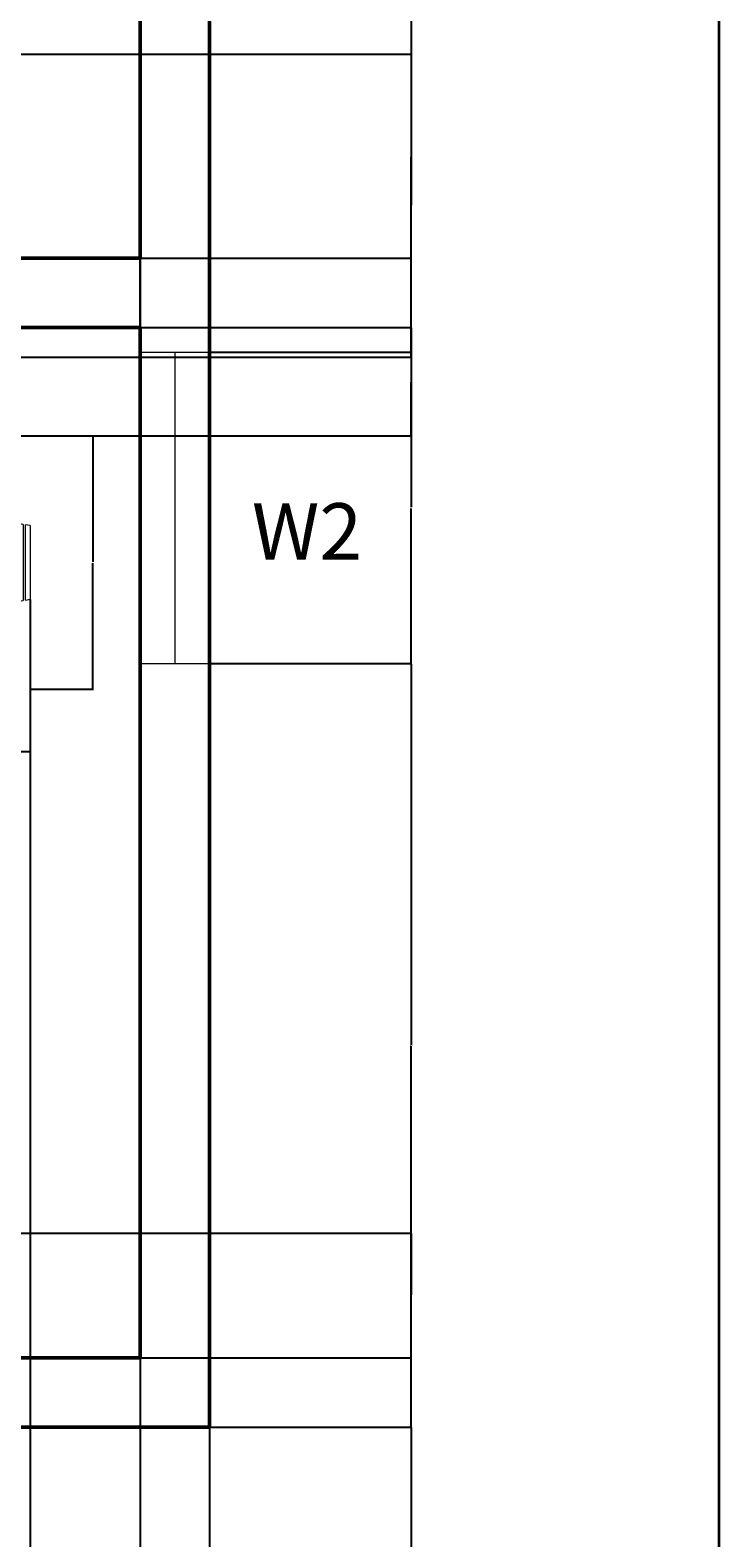
# Model space of a CAD drawing. Units: centimetres. Extents: x 2050 to 3144, y 831 to 2296.
# Tile 5 of 7: x 2916 to 3144, y 1152 to 1650. Entities that reach past the tile are written whole.
import ezdxf

# ---------------------------------------------------------------- set-up
doc = ezdxf.new("R2010")
doc.units = ezdxf.units.CM
for name, color, linetype, lineweight in [('A-ANNO-DIMS', 2, 'Continuous', 18), ('A-ANNO-TEXT', 7, 'Continuous', 18), ('A-ANNO-TTLB', 7, 'Continuous', 35), ('A-FLOR', 7, 'Continuous', 25), ('A-FURN', 8, 'Continuous', 18), ('A-GLAZ', 4, 'Continuous', 18), ('A-WALL', 7, 'Continuous', 50)]:
    doc.layers.add(name, color=color, linetype=linetype, lineweight=lineweight)
doc.styles.get("Standard").update_dxf_attribs({"font": 'arial.ttf'})
doc.dimstyles.get("Standard").update_dxf_attribs({"dimtxt": 0.18, "dimasz": 0.18, "dimexe": 0.18, "dimexo": 0.0625, "dimgap": 0.09, "dimtad": 0, "dimtih": 1, "dimtoh": 1, "dimdec": 4, "dimzin": 0, "dimdsep": 46, "dimtxsty": 'Standard', "dimcen": 0.09, "dimadec": 0, "dimazin": 0, "dimtfac": 1, "dimtdec": 4, "dimtofl": 0, "dimtmove": 0, "dimatfit": 3, "dimfxl": 1, "dimtolj": 1, "dimtzin": 0, "dimarcsym": 0})

# ---------------------------------------------------------------- blocks, each defined once
blk = doc.blocks.new('Dining Set - 36 x 72 in.')
for p, q in [((-22, 27.5), (-22.1562, 26.50042)), ((-5.8416, 26.5), (-22.1534, 26.5)), ((-22, 27.5), (-6, 27.5)), ((-5.8437, 26.49966), (-6, 27.5)), ((6, 27.5), (5.8438, 26.50042)), ((22.1584, 26.5), (5.8466, 26.5)), ((6, 27.5), (22, 27.5)), ((22.1563, 26.49966), (22, 27.5)), ((-22.2343, 26.00059), (-23.4847, 17.99762)), ((-22.2304, 26), (-5.7608, 26)), ((-4.5152, 17.99762), (-5.7655, 25.99926)), ((5.7657, 26.00059), (4.5153, 17.99762)), ((5.7696, 26), (22.2392, 26)), ((23.4848, 17.99762), (22.2345, 25.99926)), ((36, 18), (-36, 18)), ((-36, 18), (-36, -18)), ((36, -18), (36, 18)), ((-45.5, 8), (-44.5004, 8.15617)), ((-45.5, 8), (-45.5, -8)), ((-44.5, -8.15843), (-44.5, 8.15338)), ((-44.0006, 8.23428), (-35.9976, 9.48474)), ((-44, 8.23041), (-44, -8.23915)), ((44.0006, 8.23428), (35.9976, 9.48474)), ((44, 8.23041), (44, -8.23915)), ((44.5, -8.15843), (44.5, 8.15338)), ((45.5, 8), (44.5005, 8.15617)), ((45.5, 8), (45.5, -8)), ((-44.4997, -8.15631), (-45.5, -8)), ((-35.9976, -9.48476), (-43.9993, -8.2345)), ((35.9976, -9.48476), (43.9993, -8.2345)), ((44.4997, -8.15631), (45.5, -8)), ((-36, -18), (36, -18)), ((-22.2343, -26.0006), (-23.4847, -17.99762)), ((-4.5152, -17.99762), (-5.7655, -25.99928)), ((5.7657, -26.0006), (4.5153, -17.99762)), ((23.4848, -17.99762), (22.2345, -25.99928)), ((-22.2304, -26), (-5.7608, -26)), ((5.7696, -26), (22.2392, -26)), ((-22, -27.5), (-22.1562, -26.50044)), ((-5.8416, -26.5), (-22.1534, -26.5)), ((-22, -27.5), (-6, -27.5)), ((-5.8437, -26.49967), (-6, -27.5)), ((6, -27.5), (5.8438, -26.50044)), ((22.1584, -26.5), (5.8466, -26.5)), ((6, -27.5), (22, -27.5)), ((22.1563, -26.49967), (22, -27.5))]:
    blk.add_line(p, q)
for points in [[(-36, 15), (-31.1772, 14.97754), (-26.8079, 14.91406), (-22.8538, 14.81543), (-19.276, 14.6875), (-16.0362, 14.53613), (-13.0957, 14.36718), (-10.4159, 14.18652), (-7.9583, 14), (-5.6904, 13.81315), (-3.6035, 13.63021), (-1.6954, 13.45508), (0.0365, 13.29166), (1.5945, 13.14388), (2.9811, 13.01562), (4.1988, 12.9108), (5.25, 12.83333), (6.1393, 12.78613), (6.8802, 12.76823), (7.4883, 12.77767), (7.9792, 12.8125), (8.3685, 12.87077), (8.6719, 12.95052), (8.9049, 13.0498), (9.0833, 13.16666), (9.2205, 13.29899), (9.3216, 13.44401), (9.3895, 13.59879), (9.4271, 13.76041), (9.4373, 13.92594), (9.4232, 14.09245), (9.3875, 14.257), (9.3333, 14.41666), (9.2638, 14.56917), (9.1836, 14.71484), (9.0975, 14.85465), (9.0104, 14.98958), (8.9272, 15.1206), (8.8529, 15.2487), (8.7922, 15.37483), (8.75, 15.5), (8.7305, 15.62467), (8.7344, 15.74739), (8.7617, 15.86621), (8.8125, 15.97916), (8.8867, 16.08431), (8.9844, 16.17968), (9.1055, 16.26334), (9.25, 16.33333), (9.4189, 16.38802), (9.6172, 16.42708), (9.8506, 16.45052), (10.125, 16.45833), (10.4463, 16.45052), (10.8203, 16.42708), (11.2529, 16.38802), (11.75, 16.33333), (12.3184, 16.26318), (12.9694, 16.17838), (13.7151, 16.07991), (14.5677, 15.96875), (15.5395, 15.84586), (16.6426, 15.71224), (17.8893, 15.56884), (19.2917, 15.41666), (20.859, 15.25667), (22.5879, 15.08984), (24.4721, 14.91715), (26.5052, 14.73958), (28.6809, 14.5581), (30.9929, 14.3737), (33.4347, 14.18733), (36, 14)], [(-36, 10), (-28.9766, 10.14274), (-23.1725, 10.20442), (-18.4241, 10.19775), (-14.5677, 10.13541), (-11.4399, 10.03011), (-8.877, 9.89453), (-6.7154, 9.74137), (-4.7917, 9.58333), (-2.9698, 9.43082), (-1.2246, 9.28515), (0.4415, 9.14534), (2.026, 9.01041), (3.5266, 8.87939), (4.9408, 8.7513), (6.266, 8.62516), (7.5, 8.5), (8.6411, 8.37549), (9.6914, 8.2539), (10.6538, 8.13818), (11.5312, 8.03125), (12.3267, 7.93603), (13.043, 7.85547), (13.6831, 7.79248), (14.25, 7.75), (14.7471, 7.7303), (15.1797, 7.73307), (15.5537, 7.75732), (15.875, 7.80208), (16.1494, 7.86637), (16.3828, 7.94922), (16.5811, 8.04964), (16.75, 8.16666), (16.8944, 8.29915), (17.0143, 8.44531), (17.1089, 8.60319), (17.1771, 8.77083), (17.218, 8.94629), (17.2305, 9.1276), (17.2137, 9.31282), (17.1667, 9.5), (17.0895, 9.6875), (16.987, 9.875), (16.8649, 10.0625), (16.7292, 10.25), (16.5856, 10.4375), (16.4401, 10.625), (16.2985, 10.8125), (16.1667, 11), (16.05, 11.18733), (15.9518, 11.3737), (15.8752, 11.5581), (15.8229, 11.73958), (15.798, 11.91715), (15.8034, 12.08984), (15.842, 12.25667), (15.9167, 12.41666), (16.0295, 12.56836), (16.1784, 12.70833), (16.3605, 12.83268), (16.5729, 12.9375), (16.8127, 13.01888), (17.0768, 13.07291), (17.3625, 13.0957), (17.6667, 13.08333), (17.9894, 13.03312), (18.3418, 12.94726), (18.7382, 12.82918), (19.1927, 12.68229), (19.7195, 12.51001), (20.3327, 12.31575), (21.0465, 12.10294), (21.875, 11.875), (22.8357, 11.63354), (23.959, 11.37304), (25.2786, 11.08618), (26.8282, 10.76562), (28.6414, 10.40405), (30.752, 9.99414), (33.1936, 9.52856), (36, 9)], [(-36, 5.5), (-30.7157, 5.3348), (-26.069, 5.20963), (-21.9946, 5.11767), (-18.4271, 5.05208), (-15.3009, 5.00602), (-12.5508, 4.97265), (-10.1112, 4.94515), (-7.9167, 4.91666), (-5.909, 4.88167), (-4.0586, 4.83984), (-2.3429, 4.79215), (-0.7396, 4.73958), (0.7739, 4.6831), (2.22, 4.6237), (3.6213, 4.56233), (5, 4.5), (6.373, 4.43782), (7.7344, 4.3776), (9.0723, 4.32129), (10.375, 4.27083), (11.6309, 4.22819), (12.8281, 4.19531), (13.9551, 4.17415), (15, 4.16666), (15.954, 4.17448), (16.819, 4.19791), (17.6001, 4.23698), (18.3021, 4.29166), (18.9299, 4.36198), (19.4883, 4.44791), (19.9823, 4.54948), (20.4167, 4.66666), (20.7969, 4.79899), (21.1302, 4.94401), (21.4245, 5.09879), (21.6875, 5.26041), (21.9271, 5.42594), (22.1511, 5.59245), (22.3672, 5.757), (22.5834, 5.91666), (22.8065, 6.06868), (23.0404, 6.21093), (23.2879, 6.34147), (23.5521, 6.45833), (23.8358, 6.55957), (24.142, 6.64323), (24.4735, 6.70735), (24.8334, 6.75), (25.2235, 6.76969), (25.642, 6.76692), (26.0858, 6.74267), (26.5521, 6.69791), (27.0379, 6.63362), (27.5404, 6.55078), (28.0565, 6.45036), (28.5834, 6.33333), (29.1242, 6.19987), (29.7071, 6.04687), (30.3661, 5.87044), (31.1354, 5.66666), (32.0493, 5.43164), (33.142, 5.16146), (34.4475, 4.85221), (36, 4.5)], [(-36, -1), (-30.7915, -0.6591), (-26.0195, -0.38216), (-21.6519, -0.16284), (-17.6563, 0.00521), (-14.0005, 0.12833), (-10.6523, 0.21289), (-7.5796, 0.26522), (-4.75, 0.29166), (-2.134, 0.29793), (0.2878, 0.28711), (2.5317, 0.26163), (4.6146, 0.22396), (6.5529, 0.17651), (8.3633, 0.12174), (10.0623, 0.06209), (11.6667, 0), (13.1899, -0.06201), (14.6341, -0.1211), (15.9982, -0.17432), (17.2813, -0.21875), (18.4823, -0.25147), (19.6003, -0.26953), (20.6343, -0.27002), (21.5834, -0.25), (22.4481, -0.20768), (23.2357, -0.14584), (23.9549, -0.06836), (24.6146, 0.02083), (25.2235, 0.11784), (25.7904, 0.21875), (26.3241, 0.31966), (26.8334, 0.41666), (27.3265, 0.50618), (27.8099, 0.58593), (28.2894, 0.65397), (28.7709, 0.70833), (29.2601, 0.74707), (29.763, 0.76823), (30.2855, 0.76985), (30.8334, 0.75), (31.4088, 0.70784), (31.9994, 0.64713), (32.589, 0.57275), (33.1615, 0.48958), (33.7008, 0.4025), (34.1908, 0.3164), (34.6153, 0.23616), (34.9584, 0.16666), (35.2099, 0.11165), (35.3848, 0.07031), (35.504, 0.04069), (35.5886, 0.02083), (35.6594, 0.00879), (35.7377, 0.0026), (35.8442, 0.00032), (36, 0)], [(-36, -6.5), (-27.1843, -6.31267), (-20.084, -6.1263), (-14.469, -5.9419), (-10.1094, -5.76042), (-6.7752, -5.58285), (-4.2363, -5.41016), (-2.2629, -5.24333), (-0.625, -5.08334), (0.8708, -4.93099), (2.2715, -4.78646), (3.5872, -4.64974), (4.8281, -4.52084), (6.0046, -4.39974), (7.127, -4.28646), (8.2053, -4.18099), (9.25, -4.08334), (10.2705, -3.99382), (11.2734, -3.91407), (12.2647, -3.84603), (13.25, -3.79167), (14.2354, -3.75293), (15.2266, -3.73177), (16.2295, -3.73015), (17.25, -3.75), (18.2912, -3.79248), (19.3451, -3.85547), (20.4009, -3.93604), (21.4479, -4.03125), (22.4754, -4.13819), (23.4727, -4.25391), (24.4289, -4.37549), (25.3334, -4.5), (26.1785, -4.62492), (26.9694, -4.74935), (27.7145, -4.87281), (28.4219, -4.99479), (29.1, -5.11483), (29.7572, -5.23242), (30.4016, -5.34709), (31.0417, -5.45834), (31.6837, -5.56437), (32.3262, -5.65821), (32.9658, -5.73153), (33.599, -5.77604), (34.2224, -5.78345), (34.8327, -5.74545), (35.4264, -5.65373), (36, -5.5)], [(-36, -10), (-26.4022, -9.81299), (-18.4675, -9.62891), (-11.9839, -9.45069), (-6.7396, -9.28125), (-2.5226, -9.12354), (0.8789, -8.98047), (3.6769, -8.85498), (6.0833, -8.75), (8.2767, -8.66765), (10.3021, -8.60677), (12.1712, -8.56543), (13.8958, -8.54167), (15.4876, -8.53353), (16.9583, -8.53907), (18.3197, -8.55632), (19.5834, -8.58334), (20.7616, -8.61841), (21.8685, -8.66081), (22.9188, -8.71004), (23.9271, -8.76563), (24.9081, -8.82707), (25.8763, -8.89388), (26.8465, -8.96558), (27.8334, -9.04167), (28.8474, -9.12118), (29.8828, -9.20117), (30.93, -9.27824), (31.9792, -9.34896), (33.0205, -9.40991), (34.0443, -9.45768), (35.0407, -9.48885), (36, -9.5)], [(-36, -14.5), (-30.0881, -14.33513), (-25.0332, -14.21224), (-20.7312, -14.12647), (-17.0781, -14.07292), (-13.97, -14.04671), (-11.3027, -14.04297), (-8.9724, -14.05681), (-6.875, -14.08334), (-4.9224, -14.11833), (-3.0905, -14.16016), (-1.3709, -14.20785), (0.2448, -14.26042), (1.7647, -14.3169), (3.1973, -14.3763), (4.5507, -14.43767), (5.8333, -14.5), (7.0554, -14.5621), (8.235, -14.62175), (9.3922, -14.67652), (10.5469, -14.72396), (11.7192, -14.76164), (12.929, -14.78711), (14.1965, -14.79794), (15.5417, -14.79167), (16.9933, -14.76424), (18.6152, -14.70508), (20.4804, -14.60197), (22.6615, -14.44271), (25.2312, -14.21509), (28.2624, -13.9069), (31.8277, -13.50594), (36, -13)]]:
    blk.add_lwpolyline(points)
blk = doc.blocks.new('*D19')
at = {"layer": 'A-ANNO-DIMS', "color": 0, "lineweight": -2, "transparency": 16777216}
for p, q in [((2778.22, 1432.48), (2778.22, 1411.63)), ((2916.44, 1432.48), (2916.44, 1411.63)), ((2778.4, 1411.81), (2846.29, 1411.81)), ((2916.26, 1411.81), (2848.37, 1411.81))]:
    blk.add_line(p, q, dxfattribs=at)
at = {"layer": 'A-ANNO-DIMS', "color": 0, "transparency": 16777216}
for points in [[(2778.4, 1411.84), (2778.4, 1411.78), (2778.22, 1411.81)], [(2916.26, 1411.84), (2916.26, 1411.78), (2916.44, 1411.81)]]:
    blk.add_solid(points, dxfattribs=at)
at = {"layer": 'Defpoints', "color": 0, "transparency": 16777216}
for p in [(2778.22, 1432.54), (2916.44, 1432.54), (2916.44, 1411.81)]:
    blk.add_point(p, dxfattribs=at)
at = {"layer": 'A-ANNO-DIMS', "color": 0, "transparency": 16777216, "insert": (2847.33, 1411.81), "char_height": 0.18, "attachment_point": 5}
blk.add_mtext('\\A1;DINING SET 138', dxfattribs=at)
blk = doc.blocks.new('*D20')
at = {"layer": 'A-ANNO-DIMS', "color": 0, "lineweight": -2, "transparency": 16777216}
for p, q in [((2916.5, 1516.08), (2937.35, 1516.08)), ((2937.17, 1515.9), (2937.17, 1474.49)), ((2937.17, 1432.72), (2937.17, 1474.13)), ((2916.5, 1432.54), (2937.35, 1432.54))]:
    blk.add_line(p, q, dxfattribs=at)
at = {"layer": 'A-ANNO-DIMS', "color": 0, "transparency": 16777216}
for points in [[(2937.14, 1515.9), (2937.2, 1515.9), (2937.17, 1516.08)], [(2937.14, 1432.72), (2937.2, 1432.72), (2937.17, 1432.54)]]:
    blk.add_solid(points, dxfattribs=at)
at = {"layer": 'Defpoints', "color": 0, "transparency": 16777216}
for p in [(2916.44, 1516.08), (2937.17, 1516.08), (2916.44, 1432.54)]:
    blk.add_point(p, dxfattribs=at)
at = {"layer": 'A-ANNO-DIMS', "color": 0, "transparency": 16777216, "insert": (2937.17, 1474.31), "char_height": 0.18, "attachment_point": 5}
blk.add_mtext('\\A1;84', dxfattribs=at)
blk = doc.blocks.new('*D43')
at = {"layer": 'A-ANNO-DIMS', "color": 0, "lineweight": -2, "transparency": 16777216}
for p, q in [((2975.65, 1440.94), (3042.37, 1440.94)), ((3042.19, 1440.76), (3042.19, 1315.16)), ((3042.19, 1189.19), (3042.19, 1314.8)), ((2975.65, 1189.01), (3042.37, 1189.01))]:
    blk.add_line(p, q, dxfattribs=at)
at = {"layer": 'A-ANNO-DIMS', "color": 0, "transparency": 16777216}
for points in [[(3042.16, 1440.76), (3042.22, 1440.76), (3042.19, 1440.94)], [(3042.16, 1189.19), (3042.22, 1189.19), (3042.19, 1189.01)]]:
    blk.add_solid(points, dxfattribs=at)
at = {"layer": 'Defpoints', "color": 0, "transparency": 16777216}
for p in [(2975.59, 1440.94), (3042.19, 1440.94), (2975.59, 1189.01)]:
    blk.add_point(p, dxfattribs=at)
at = {"layer": 'A-ANNO-DIMS', "color": 0, "transparency": 16777216, "insert": (3042.19, 1314.98), "char_height": 0.18, "attachment_point": 5}
blk.add_mtext('\\A1;251.93', dxfattribs=at)
blk = doc.blocks.new('*D44')
at = {"layer": 'A-ANNO-DIMS', "color": 0, "lineweight": -2, "transparency": 16777216}
for p, q in [((2975.65, 1543.76), (3042.37, 1543.76)), ((3042.19, 1543.58), (3042.19, 1492.53)), ((3042.19, 1441.12), (3042.19, 1492.17)), ((2975.65, 1440.94), (3042.37, 1440.94))]:
    blk.add_line(p, q, dxfattribs=at)
at = {"layer": 'A-ANNO-DIMS', "color": 0, "transparency": 16777216}
for points in [[(3042.16, 1543.58), (3042.22, 1543.58), (3042.19, 1543.76)], [(3042.16, 1441.12), (3042.22, 1441.12), (3042.19, 1440.94)]]:
    blk.add_solid(points, dxfattribs=at)
at = {"layer": 'Defpoints', "color": 0, "transparency": 16777216}
for p in [(2975.59, 1543.76), (3042.19, 1543.76), (2975.59, 1440.94)]:
    blk.add_point(p, dxfattribs=at)
at = {"layer": 'A-ANNO-DIMS', "color": 0, "transparency": 16777216, "insert": (3042.19, 1492.35), "char_height": 0.18, "attachment_point": 5}
blk.add_mtext('\\A1;102.81', dxfattribs=at)
blk = doc.blocks.new('*D45')
at = {"layer": 'A-ANNO-DIMS', "color": 0, "lineweight": -2, "transparency": 16777216}
for p, q in [((2975.65, 1663.11), (3042.37, 1663.11)), ((3042.19, 1662.93), (3042.19, 1603.62)), ((3042.19, 1543.94), (3042.19, 1603.25)), ((2975.65, 1543.76), (3042.37, 1543.76))]:
    blk.add_line(p, q, dxfattribs=at)
at = {"layer": 'A-ANNO-DIMS', "color": 0, "transparency": 16777216}
for points in [[(3042.16, 1662.93), (3042.22, 1662.93), (3042.19, 1663.11)], [(3042.16, 1543.94), (3042.22, 1543.94), (3042.19, 1543.76)]]:
    blk.add_solid(points, dxfattribs=at)
at = {"layer": 'Defpoints', "color": 0, "transparency": 16777216}
for p in [(2975.59, 1663.11), (3042.19, 1663.11), (2975.59, 1543.76)]:
    blk.add_point(p, dxfattribs=at)
at = {"layer": 'A-ANNO-DIMS', "color": 0, "transparency": 16777216, "insert": (3042.19, 1603.43), "char_height": 0.18, "attachment_point": 5}
blk.add_mtext('\\A1;119.36', dxfattribs=at)
blk = doc.blocks.new('*D52')
at = {"layer": 'A-ANNO-DIMS', "color": 0, "lineweight": -2, "transparency": 16777216}
for p, q in [((2513.42, 1642.03), (3042.37, 1642.03)), ((3042.19, 1641.85), (3042.19, 1592.22)), ((3042.19, 1542.21), (3042.19, 1591.85)), ((2513.42, 1542.03), (3042.37, 1542.03))]:
    blk.add_line(p, q, dxfattribs=at)
at = {"layer": 'A-ANNO-DIMS', "color": 0, "transparency": 16777216}
for points in [[(3042.16, 1641.85), (3042.22, 1641.85), (3042.19, 1642.03)], [(3042.16, 1542.21), (3042.22, 1542.21), (3042.19, 1542.03)]]:
    blk.add_solid(points, dxfattribs=at)
at = {"layer": 'Defpoints', "color": 0, "transparency": 16777216}
for p in [(2513.36, 1642.03), (3042.19, 1642.03), (2513.36, 1542.03)]:
    blk.add_point(p, dxfattribs=at)
at = {"layer": 'A-ANNO-DIMS', "color": 0, "transparency": 16777216, "insert": (3042.19, 1592.03), "char_height": 0.18, "attachment_point": 5}
blk.add_mtext('\\A1;100', dxfattribs=at)
blk = doc.blocks.new('*D56')
at = {"layer": 'A-ANNO-DIMS', "color": 0, "lineweight": -2, "transparency": 16777216}
for p, q in [((2652.79, 1642.03), (3042.37, 1642.03)), ((3042.19, 1641.85), (3042.19, 1608.57)), ((3042.19, 1574.91), (3042.19, 1608.2)), ((2630.24, 1574.73), (3042.37, 1574.73))]:
    blk.add_line(p, q, dxfattribs=at)
at = {"layer": 'A-ANNO-DIMS', "color": 0, "transparency": 16777216}
for points in [[(3042.16, 1641.85), (3042.22, 1641.85), (3042.19, 1642.03)], [(3042.16, 1574.91), (3042.22, 1574.91), (3042.19, 1574.73)]]:
    blk.add_solid(points, dxfattribs=at)
at = {"layer": 'Defpoints', "color": 0, "transparency": 16777216}
for p in [(2652.73, 1642.03), (2630.18, 1574.73), (3042.19, 1574.73)]:
    blk.add_point(p, dxfattribs=at)
at = {"layer": 'A-ANNO-DIMS', "color": 0, "transparency": 16777216, "insert": (3042.19, 1608.38), "char_height": 0.18, "attachment_point": 5}
blk.add_mtext('\\A1;67.3', dxfattribs=at)
blk = doc.blocks.new('*D57')
at = {"layer": 'A-ANNO-DIMS', "color": 0, "lineweight": -2, "transparency": 16777216}
for p, q in [((2916.44, 1462.1), (2916.44, 1009.53)), ((2952.73, 1440.88), (2952.73, 1009.53)), ((2916.62, 1009.71), (2934.19, 1009.71)), ((2952.55, 1009.71), (2934.98, 1009.71))]:
    blk.add_line(p, q, dxfattribs=at)
at = {"layer": 'A-ANNO-DIMS', "color": 0, "transparency": 16777216}
for points in [[(2916.62, 1009.74), (2916.62, 1009.68), (2916.44, 1009.71)], [(2952.55, 1009.74), (2952.55, 1009.68), (2952.73, 1009.71)]]:
    blk.add_solid(points, dxfattribs=at)
at = {"layer": 'Defpoints', "color": 0, "transparency": 16777216}
for p in [(2916.44, 1462.16), (2952.73, 1440.94), (2952.73, 1009.71)]:
    blk.add_point(p, dxfattribs=at)
at = {"layer": 'A-ANNO-DIMS', "color": 0, "transparency": 16777216, "insert": (2934.58, 1009.71), "char_height": 0.18, "attachment_point": 5}
blk.add_mtext('\\A1;36.29', dxfattribs=at)
blk = doc.blocks.new('*D58')
at = {"layer": 'A-ANNO-DIMS', "color": 0, "lineweight": -2, "transparency": 16777216}
for p, q in [((2952.79, 1551.87), (3042.37, 1551.87)), ((3042.19, 1551.69), (3042.19, 1534.16)), ((3042.19, 1516.26), (3042.19, 1533.8)), ((2838.28, 1516.08), (3042.37, 1516.08))]:
    blk.add_line(p, q, dxfattribs=at)
at = {"layer": 'A-ANNO-DIMS', "color": 0, "transparency": 16777216}
for points in [[(3042.16, 1551.69), (3042.22, 1551.69), (3042.19, 1551.87)], [(3042.16, 1516.26), (3042.22, 1516.26), (3042.19, 1516.08)]]:
    blk.add_solid(points, dxfattribs=at)
at = {"layer": 'Defpoints', "color": 0, "transparency": 16777216}
for p in [(2952.73, 1551.87), (3042.19, 1551.87), (2838.22, 1516.08)]:
    blk.add_point(p, dxfattribs=at)
at = {"layer": 'A-ANNO-DIMS', "color": 0, "transparency": 16777216, "insert": (3042.19, 1533.98), "char_height": 0.18, "attachment_point": 5}
blk.add_mtext('\\A1;35.794', dxfattribs=at)
blk = doc.blocks.new('*D59')
at = {"layer": 'A-ANNO-DIMS', "color": 0, "lineweight": -2, "transparency": 16777216}
for p, q in [((2862.15, 1253.11), (2862.15, 2154.53)), ((2862.33, 2154.35), (2907.04, 2154.35)), ((2952.55, 2154.35), (2907.83, 2154.35)), ((2952.73, 1211.94), (2952.73, 2154.53))]:
    blk.add_line(p, q, dxfattribs=at)
at = {"layer": 'A-ANNO-DIMS', "color": 0, "transparency": 16777216}
for points in [[(2862.33, 2154.38), (2862.33, 2154.32), (2862.15, 2154.35)], [(2952.55, 2154.38), (2952.55, 2154.32), (2952.73, 2154.35)]]:
    blk.add_solid(points, dxfattribs=at)
at = {"layer": 'Defpoints', "color": 0, "transparency": 16777216}
for p in [(2952.73, 2154.35), (2862.15, 1253.05), (2952.73, 1211.87)]:
    blk.add_point(p, dxfattribs=at)
at = {"layer": 'A-ANNO-DIMS', "color": 0, "transparency": 16777216, "insert": (2907.44, 2154.35), "char_height": 0.18, "attachment_point": 5}
blk.add_mtext('\\A1;90.58', dxfattribs=at)
blk = doc.blocks.new('*D60')
at = {"layer": 'A-ANNO-DIMS', "color": 0, "lineweight": -2, "transparency": 16777216}
for p, q in [((2862.21, 1253.05), (3042.37, 1253.05)), ((3042.19, 1252.87), (3042.19, 1232.65)), ((3042.19, 1212.05), (3042.19, 1232.28)), ((2895.42, 1211.87), (3042.37, 1211.87))]:
    blk.add_line(p, q, dxfattribs=at)
at = {"layer": 'A-ANNO-DIMS', "color": 0, "transparency": 16777216}
for points in [[(3042.16, 1252.87), (3042.22, 1252.87), (3042.19, 1253.05)], [(3042.16, 1212.05), (3042.22, 1212.05), (3042.19, 1211.87)]]:
    blk.add_solid(points, dxfattribs=at)
at = {"layer": 'Defpoints', "color": 0, "transparency": 16777216}
for p in [(2862.15, 1253.05), (2895.36, 1211.87), (3042.19, 1211.87)]:
    blk.add_point(p, dxfattribs=at)
at = {"layer": 'A-ANNO-DIMS', "color": 0, "transparency": 16777216, "insert": (3042.19, 1232.46), "char_height": 0.18, "attachment_point": 5}
blk.add_mtext('\\A1;41.18', dxfattribs=at)
blk = doc.blocks.new('*D64')
at = {"layer": 'A-ANNO-DIMS', "color": 0, "lineweight": -2, "transparency": 16777216}
for p, q in [((2975.65, 1189.01), (3042.37, 1189.01)), ((3042.19, 1188.83), (3042.19, 1132.85)), ((3042.19, 1076.49), (3042.19, 1132.48)), ((2975.65, 1076.31), (3042.37, 1076.31))]:
    blk.add_line(p, q, dxfattribs=at)
at = {"layer": 'A-ANNO-DIMS', "color": 0, "transparency": 16777216}
for points in [[(3042.16, 1188.83), (3042.22, 1188.83), (3042.19, 1189.01)], [(3042.16, 1076.49), (3042.22, 1076.49), (3042.19, 1076.31)]]:
    blk.add_solid(points, dxfattribs=at)
at = {"layer": 'Defpoints', "color": 0, "transparency": 16777216}
for p in [(2975.59, 1189.01), (3042.19, 1189.01), (2975.59, 1076.31)]:
    blk.add_point(p, dxfattribs=at)
at = {"layer": 'A-ANNO-DIMS', "color": 0, "transparency": 16777216, "insert": (3042.19, 1132.66), "char_height": 0.18, "attachment_point": 5}
blk.add_mtext('\\A1;112.7', dxfattribs=at)
blk = doc.blocks.new('*D74')
at = {"layer": 'A-ANNO-DIMS', "color": 0, "lineweight": -2, "transparency": 16777216}
for p, q in [((2952.73, 2064.83), (2952.73, 1009.53)), ((2822.89, 2004.16), (2822.89, 1009.53)), ((2823.07, 1009.71), (2887.35, 1009.71)), ((2952.55, 1009.71), (2888.26, 1009.71))]:
    blk.add_line(p, q, dxfattribs=at)
at = {"layer": 'A-ANNO-DIMS', "color": 0, "transparency": 16777216}
for points in [[(2823.07, 1009.74), (2823.07, 1009.68), (2822.89, 1009.71)], [(2952.55, 1009.74), (2952.55, 1009.68), (2952.73, 1009.71)]]:
    blk.add_solid(points, dxfattribs=at)
at = {"layer": 'Defpoints', "color": 0, "transparency": 16777216}
for p in [(2952.73, 2064.89), (2822.89, 2004.22), (2952.73, 1009.71)]:
    blk.add_point(p, dxfattribs=at)
at = {"layer": 'A-ANNO-DIMS', "color": 0, "transparency": 16777216, "insert": (2887.81, 1009.71), "char_height": 0.18, "attachment_point": 5}
blk.add_mtext('\\A1;129.84', dxfattribs=at)

msp = doc.modelspace()

# ---------------------------------------------------------------- linework, layer by layer
at = {"layer": 'A-ANNO-TTLB'}
msp.add_lwpolyline([(2050.3641, 2295.8578), (3143.7558, 2295.8578), (3143.7558, 830.6902), (2050.3641, 830.6902)], close=True, dxfattribs=at)
at = {"layer": 'A-FLOR'}
msp.add_line((2975.5865, 1551.8748), (2975.5865, 1076.3148), dxfattribs=at)
at = {"layer": 'A-GLAZ'}
for p, q in [((2952.7265, 1543.7558), (2975.5865, 1543.7558)), ((2964.1565, 1543.7558), (2964.1565, 1440.9424)), ((2952.7265, 1440.9424), (2975.5865, 1440.9424))]:
    msp.add_line(p, q, dxfattribs=at)
at = {"layer": 'A-WALL'}
for p, q in [((2952.7265, 1914.7348), (2952.7265, 1574.7348)), ((2975.5865, 1914.7348), (2975.5865, 1189.0148)), ((2952.7265, 1574.7348), (2629.8665, 1574.7348)), ((2952.7265, 1574.7348), (2952.7265, 1574.7348)), ((2952.7265, 1551.8748), (2629.8665, 1551.8748)), ((2952.7265, 1551.8748), (2952.7265, 1211.8748)), ((2952.7265, 1211.8748), (2669.2319, 1211.8748)), ((2975.5865, 1189.0148), (2669.2319, 1189.0148))]:
    msp.add_line(p, q, dxfattribs=at)

# ---------------------------------------------------------------- block references
at = {"layer": 'A-FURN', "xscale": 1.518878716440213, "yscale": 1.518878716440213, "zscale": 1.518878716440213}
msp.add_blockref('Dining Set - 36 x 72 in.', (2847.3285, 1474.3117), dxfattribs=at)

# ---------------------------------------------------------------- texts
at = {"layer": 'A-ANNO-TEXT'}
msp.add_text('W2', height=18.59595, dxfattribs=at).set_placement((2989.6243, 1475.2678))

# ---------------------------------------------------------------- dimensions: what is measured, and where the dimension line sits
at = {"layer": 'A-ANNO-DIMS'}
for base, p1, p2, picture, middle in [((2952.7265, 2154.3548), (2862.1454, 1253.0515), (2952.7265, 1211.8748), '*D59', (2907.436, 2154.3548)), ((2952.7265, 1009.7148), (2822.8865, 2004.2202), (2952.7265, 2064.8948), '*D74', (2887.8065, 1009.7148)), ((2952.7265, 1009.7148), (2916.4375, 1462.1606), (2952.7265, 1440.9424), '*D57', (2934.582, 1009.7148))]:
    dim = msp.add_linear_dim(base=base, p1=p1, p2=p2, dimstyle='Standard', override={"dimdec": 2, "dimlfac": 1, "dimrnd": 0, "dimzin": 0, "dimdsep": 46, "dimlunit": 2}, dxfattribs=at)
    dim.commit()
    dim.dimension.update_dxf_attribs({"geometry": picture, "text_midpoint": middle})
for base, p1, p2, override, picture, middle in [((3042.1865, 1663.1111), (2975.5865, 1543.7558), (2975.5865, 1663.1111), {"dimdec": 2, "dimlfac": 1, "dimrnd": 0, "dimzin": 0, "dimdsep": 46, "dimlunit": 2}, '*D45', (3042.1865, 1603.4335)), ((3042.1865, 1642.0348), (2513.3612, 1542.0348), (2513.3612, 1642.0348), {"dimdec": 0, "dimlfac": 1, "dimrnd": 0, "dimzin": 0, "dimdsep": 46, "dimlunit": 2}, '*D52', (3042.1865, 1592.0348)), ((3042.1865, 1574.7348), (2652.7265, 1642.0348), (2630.1795, 1574.7348), {"dimdec": 1, "dimlfac": 1, "dimrnd": 0, "dimzin": 0, "dimdsep": 46, "dimlunit": 2}, '*D56', (3042.1865, 1608.3848)), ((3042.1865, 1551.8748), (2838.2153, 1516.0808), (2952.7265, 1551.8748), {"dimdec": 3, "dimlfac": 1, "dimrnd": 0, "dimzin": 0, "dimdsep": 46, "dimlunit": 2}, '*D58', (3042.1865, 1533.9778)), ((3042.1865, 1543.7558), (2975.5865, 1440.9424), (2975.5865, 1543.7558), {"dimdec": 2, "dimlfac": 1, "dimrnd": 0, "dimzin": 0, "dimdsep": 46, "dimlunit": 2}, '*D44', (3042.1865, 1492.3491)), ((2937.1702, 1516.0808), (2916.4375, 1432.5425), (2916.4375, 1516.0808), {"dimdec": 0, "dimlfac": 1, "dimrnd": 0, "dimzin": 0, "dimdsep": 46, "dimlunit": 2}, '*D20', (2937.1702, 1474.3117)), ((3042.1865, 1440.9424), (2975.5865, 1189.0148), (2975.5865, 1440.9424), {"dimdec": 2, "dimlfac": 1, "dimrnd": 0, "dimzin": 0, "dimdsep": 46, "dimlunit": 2}, '*D43', (3042.1865, 1314.9786)), ((3042.1865, 1211.8748), (2862.1454, 1253.0515), (2895.3598, 1211.8748), {"dimdec": 2, "dimlfac": 1, "dimrnd": 0, "dimzin": 0, "dimdsep": 46, "dimlunit": 2}, '*D60', (3042.1865, 1232.4632)), ((3042.1865, 1189.0148), (2975.5865, 1076.3148), (2975.5865, 1189.0148), {"dimdec": 1, "dimlfac": 1, "dimrnd": 0, "dimzin": 0, "dimdsep": 46, "dimlunit": 2}, '*D64', (3042.1865, 1132.6648))]:
    dim = msp.add_linear_dim(base=base, p1=p1, p2=p2, angle=90, dimstyle='Standard', override=override, dxfattribs=at)
    dim.commit()
    dim.dimension.update_dxf_attribs({"geometry": picture, "text_midpoint": middle})
dim = msp.add_linear_dim(base=(2916.4375, 1411.8098), p1=(2778.2196, 1432.5425), p2=(2916.4375, 1432.5425), text='DINING SET <>', dimstyle='Standard', override={"dimdec": 0, "dimlfac": 1, "dimrnd": 0, "dimzin": 0, "dimdsep": 46, "dimlunit": 2}, dxfattribs=at)
dim.commit()
dim.dimension.update_dxf_attribs({"geometry": '*D19', "text_midpoint": (2847.3285, 1411.8098)})

doc.saveas('drawing.dxf')
